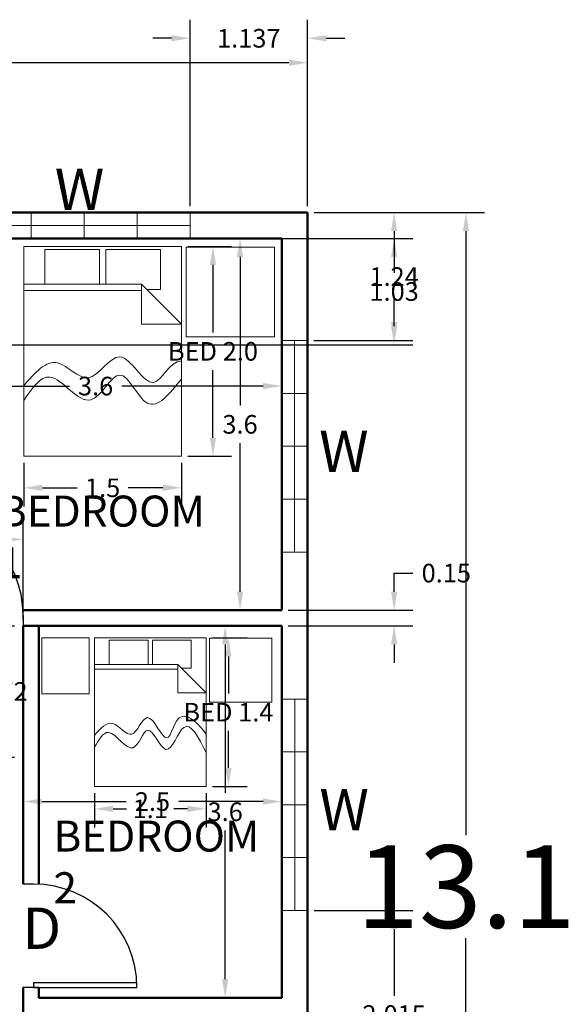
# Model space of a CAD drawing. Units: metres. Extents: x 3.9 to 21.3, y 24.8 to 56.5.
# Tile 6 of 6: x 13 to 18.3, y 31.2 to 40.8. Entities that reach past the tile are written whole.
import ezdxf

# ---------------------------------------------------------------- set-up
doc = ezdxf.new("R2010")
doc.units = ezdxf.units.M
doc.header["$MEASUREMENT"] = 0
for name, color, linetype, lineweight in [('A-AREA-IDEN', 3, 'Continuous', 25), ('DIMENSIONS', 2, 'Continuous', 18), ('DOOR', 5, 'Continuous', 25), ('FURNITURE', 6, 'Continuous', 18), ('TEXT', 3, 'Continuous', 18), ('WALL', 1, 'Continuous', 50), ('WINDOW', 4, 'Continuous', 18)]:
    doc.layers.add(name, color=color, linetype=linetype, lineweight=lineweight)
doc.styles.get("Standard").update_dxf_attribs({"font": 'arial.ttf'})
doc.dimstyles.get("Standard").update_dxf_attribs({"dimtxt": 0.18, "dimasz": 0.18, "dimexe": 0.18, "dimexo": 0.0625, "dimgap": 0.09, "dimtad": 0, "dimtih": 1, "dimtoh": 1, "dimdec": 1, "dimzin": 0, "dimdsep": 46, "dimtxsty": 'Standard', "dimcen": 0.09, "dimadec": 0, "dimazin": 0, "dimtfac": 1, "dimtdec": 1, "dimtofl": 0, "dimtmove": 0, "dimatfit": 3, "dimfxl": 1, "dimtolj": 1, "dimtzin": 0, "dimarcsym": 0})

# ---------------------------------------------------------------- blocks, each defined once
blk = doc.blocks.new('*U2')
for p, q in [((0, 0), (0, -100)), ((1000, 0), (1000, -100))]:
    blk.add_line(p, q)
blk.add_lwpolyline([(0, 0), (0, 1000), (43.75, 1000), (43.75, 0)], close=True)
blk.add_arc((0, 0), 1000, 0, 90)
blk = doc.blocks.new('Bed - Queen')
for p, q in [((0, -80.00003), (0, 0)), ((0, 0), (59.99999, 0)), ((59.99999, 0), (59.99999, -80.00003)), ((7.99999, -1.2), (28.79998, -1.2)), ((7.99999, -14.4), (7.99999, -1.2)), ((28.79998, -1.2), (28.79998, -14.4)), ((31.19999, -1.2), (51.99999, -1.2)), ((31.19999, -14.4), (31.19999, -1.2)), ((51.99999, -1.2), (51.99999, -16.4)), ((0, -14.4), (44.8, -14.4)), ((59.99999, -29.6), (44.8, -14.4)), ((44.8, -14.4), (44.8, -29.6)), ((44.8, -16.8), (0, -16.8)), ((51.99999, -16.4), (46.79936, -16.4)), ((44.8, -29.6), (59.99999, -29.6)), ((59.99999, -80.00003), (0, -80.00003))]:
    blk.add_line(p, q)
blk = doc.blocks.new('*U10')
for p, q in [((0, 0), (0, -100)), ((-1000, 0), (-1000, -100))]:
    blk.add_line(p, q)
blk.add_lwpolyline([(0, 0), (0, 1000), (-43.75, 1000), (-43.75, 0)], close=True)
blk.add_arc((0, 0), 1000, 90, 180)
blk = doc.blocks.new('*D21')
at = {"layer": 'Defpoints', "color": 0, "transparency": 16777216}
for p in [(15.7571, 38.8951), (15.7571, 25.8451), (17.2883, 25.8451)]:
    blk.add_point(p, dxfattribs=at)
at = {"layer": 'DIMENSIONS', "color": 0, "lineweight": -2, "transparency": 16777216}
for p, q in [((15.8196, 38.8951), (17.4683, 38.8951)), ((17.2883, 38.7151), (17.2883, 32.8688)), ((17.2883, 26.0251), (17.2883, 31.8713)), ((15.8196, 25.8451), (17.4683, 25.8451))]:
    blk.add_line(p, q, dxfattribs=at)
at = {"layer": 'DIMENSIONS', "color": 0, "transparency": 16777216}
for points in [[(17.2583, 38.7151), (17.3183, 38.7151), (17.2883, 38.8951)], [(17.2583, 26.0251), (17.3183, 26.0251), (17.2883, 25.8451)]]:
    blk.add_solid(points, dxfattribs=at)
at = {"layer": 'DIMENSIONS', "color": 0, "transparency": 16777216, "insert": (17.2883, 32.3701), "char_height": 0.18, "attachment_point": 5}
blk.add_mtext('\\A1;{\\H4.44444x;13.1}', dxfattribs=at)
blk = doc.blocks.new('*D22')
at = {"layer": 'Defpoints', "color": 0, "transparency": 16777216}
for p in [(15.7571, 40.3451), (6.1571, 38.8951), (15.7571, 38.8951)]:
    blk.add_point(p, dxfattribs=at)
at = {"layer": 'DIMENSIONS', "color": 0, "lineweight": -2, "transparency": 16777216}
for p, q in [((6.1571, 38.9576), (6.1571, 40.5251)), ((15.7571, 38.9576), (15.7571, 40.5251)), ((6.3371, 40.3451), (10.1392, 40.3451)), ((15.5771, 40.3451), (11.7751, 40.3451))]:
    blk.add_line(p, q, dxfattribs=at)
at = {"layer": 'DIMENSIONS', "color": 0, "transparency": 16777216}
for points in [[(6.3371, 40.3751), (6.3371, 40.3151), (6.1571, 40.3451)], [(15.5771, 40.3751), (15.5771, 40.3151), (15.7571, 40.3451)]]:
    blk.add_solid(points, dxfattribs=at)
at = {"layer": 'DIMENSIONS', "color": 0, "transparency": 16777216, "insert": (10.9571, 40.3451), "char_height": 0.18, "attachment_point": 5}
blk.add_mtext('\\A1;{\\H4.44444x;9.6}', dxfattribs=at)
blk = doc.blocks.new('*D25')
at = {"layer": 'Defpoints', "color": 0, "transparency": 16777216}
for p in [(11.9071, 37.772), (15.5071, 37.772), (15.5071, 37.2152)]:
    blk.add_point(p, dxfattribs=at)
at = {"layer": 'DIMENSIONS', "color": 0, "lineweight": -2, "transparency": 16777216}
for p, q in [((11.9071, 37.7095), (11.9071, 37.0352)), ((15.5071, 37.7095), (15.5071, 37.0352)), ((12.0871, 37.2152), (13.4534, 37.2152)), ((15.3271, 37.2152), (13.9609, 37.2152))]:
    blk.add_line(p, q, dxfattribs=at)
at = {"layer": 'DIMENSIONS', "color": 0, "transparency": 16777216}
for points in [[(12.0871, 37.2452), (12.0871, 37.1852), (11.9071, 37.2152)], [(15.3271, 37.2452), (15.3271, 37.1852), (15.5071, 37.2152)]]:
    blk.add_solid(points, dxfattribs=at)
at = {"layer": 'DIMENSIONS', "color": 0, "transparency": 16777216, "insert": (13.7071, 37.2152), "char_height": 0.18, "attachment_point": 5}
blk.add_mtext('\\A1;3.6', dxfattribs=at)
blk = doc.blocks.new('*D26')
at = {"layer": 'Defpoints', "color": 0, "transparency": 16777216}
for p in [(14.878, 38.6451), (14.9391, 35.0451), (15.1038, 35.0451)]:
    blk.add_point(p, dxfattribs=at)
at = {"layer": 'DIMENSIONS', "color": 0, "lineweight": -2, "transparency": 16777216}
for p, q in [((14.9405, 38.6451), (15.2838, 38.6451)), ((15.1038, 38.4651), (15.1038, 37.027)), ((15.1038, 35.2251), (15.1038, 36.6631)), ((15.0016, 35.0451), (15.2838, 35.0451))]:
    blk.add_line(p, q, dxfattribs=at)
at = {"layer": 'DIMENSIONS', "color": 0, "transparency": 16777216}
for points in [[(15.0738, 38.4651), (15.1338, 38.4651), (15.1038, 38.6451)], [(15.0738, 35.2251), (15.1338, 35.2251), (15.1038, 35.0451)]]:
    blk.add_solid(points, dxfattribs=at)
at = {"layer": 'DIMENSIONS', "color": 0, "transparency": 16777216, "insert": (15.1038, 36.8451), "char_height": 0.18, "attachment_point": 5}
blk.add_mtext('\\A1;3.6', dxfattribs=at)
blk = doc.blocks.new('*D28')
at = {"layer": 'Defpoints', "color": 0, "transparency": 16777216}
for p in [(13.0071, 33.4184), (15.5071, 33.4184), (13.0071, 33.1938)]:
    blk.add_point(p, dxfattribs=at)
at = {"layer": 'DIMENSIONS', "color": 0, "lineweight": -2, "transparency": 16777216}
for p, q in [((13.0071, 33.3559), (13.0071, 33.0138)), ((15.5071, 33.3559), (15.5071, 33.0138)), ((13.1871, 33.1938), (14.0011, 33.1938)), ((15.3271, 33.1938), (14.5132, 33.1938))]:
    blk.add_line(p, q, dxfattribs=at)
at = {"layer": 'DIMENSIONS', "color": 0, "transparency": 16777216}
for points in [[(13.1871, 33.2238), (13.1871, 33.1638), (13.0071, 33.1938)], [(15.3271, 33.2238), (15.3271, 33.1638), (15.5071, 33.1938)]]:
    blk.add_solid(points, dxfattribs=at)
at = {"layer": 'DIMENSIONS', "color": 0, "transparency": 16777216, "insert": (14.2571, 33.1938), "char_height": 0.18, "attachment_point": 5}
blk.add_mtext('\\A1;2.5', dxfattribs=at)
blk = doc.blocks.new('*D29')
at = {"layer": 'Defpoints', "color": 0, "transparency": 16777216}
for p in [(15.5071, 34.8951), (14.9602, 31.2951), (15.5071, 31.2951)]:
    blk.add_point(p, dxfattribs=at)
at = {"layer": 'DIMENSIONS', "color": 0, "lineweight": -2, "transparency": 16777216}
for p, q in [((15.4446, 34.8951), (14.7802, 34.8951)), ((14.9602, 34.7151), (14.9602, 33.277)), ((14.9602, 31.4751), (14.9602, 32.9131)), ((15.4446, 31.2951), (14.7802, 31.2951))]:
    blk.add_line(p, q, dxfattribs=at)
at = {"layer": 'DIMENSIONS', "color": 0, "transparency": 16777216}
for points in [[(14.9302, 34.7151), (14.9902, 34.7151), (14.9602, 34.8951)], [(14.9302, 31.4751), (14.9902, 31.4751), (14.9602, 31.2951)]]:
    blk.add_solid(points, dxfattribs=at)
at = {"layer": 'DIMENSIONS', "color": 0, "transparency": 16777216, "insert": (14.9602, 33.0951), "char_height": 0.18, "attachment_point": 5}
blk.add_mtext('\\A1;3.6', dxfattribs=at)
blk = doc.blocks.new('WIN-4-LIGHT-2046')
for p, q in [((0.5115, -0.125), (0, -0.125)), ((0.5115, -0.125), (1.0231, -0.125)), ((1.5346, -0.125), (1.0231, -0.125)), ((1.5346, -0.125), (2.0462, -0.125))]:
    blk.add_line(p, q)
for points in [[(0.5115, 0), (0, 0), (0, -0.25), (0.5115, -0.25)], [(0.5115, 0), (1.0231, 0), (1.0231, -0.25), (0.5115, -0.25)], [(1.5346, 0), (1.0231, 0), (1.0231, -0.25), (1.5346, -0.25)], [(1.5346, 0), (2.0462, 0), (2.0462, -0.25), (1.5346, -0.25)]]:
    blk.add_lwpolyline(points, close=True)
blk = doc.blocks.new('*D39')
at = {"layer": 'Defpoints', "color": 0, "transparency": 16777216}
for p in [(14.537, 38.5674), (14.8418, 38.5674), (14.537, 36.5354)]:
    blk.add_point(p, dxfattribs=at)
at = {"layer": 'DIMENSIONS', "color": 0, "lineweight": -2, "transparency": 16777216}
for p, q in [((14.5995, 38.5674), (15.0218, 38.5674)), ((14.8418, 38.3874), (14.8418, 37.7333)), ((14.8418, 36.7154), (14.8418, 37.3695)), ((14.5995, 36.5354), (15.0218, 36.5354))]:
    blk.add_line(p, q, dxfattribs=at)
at = {"layer": 'DIMENSIONS', "color": 0, "transparency": 16777216}
for points in [[(14.8118, 38.3874), (14.8718, 38.3874), (14.8418, 38.5674)], [(14.8118, 36.7154), (14.8718, 36.7154), (14.8418, 36.5354)]]:
    blk.add_solid(points, dxfattribs=at)
at = {"layer": 'DIMENSIONS', "color": 0, "transparency": 16777216, "insert": (14.8418, 37.5514), "char_height": 0.18, "attachment_point": 5}
blk.add_mtext('\\A1;BED 2.0', dxfattribs=at)
blk = doc.blocks.new('*D40')
at = {"layer": 'Defpoints', "color": 0, "transparency": 16777216}
for p in [(13.013, 36.5354), (14.537, 36.5354), (14.537, 36.2306)]:
    blk.add_point(p, dxfattribs=at)
at = {"layer": 'DIMENSIONS', "color": 0, "lineweight": -2, "transparency": 16777216}
for p, q in [((13.013, 36.4729), (13.013, 36.0506)), ((14.537, 36.4729), (14.537, 36.0506)), ((13.193, 36.2306), (13.529, 36.2306)), ((14.357, 36.2306), (14.0211, 36.2306))]:
    blk.add_line(p, q, dxfattribs=at)
at = {"layer": 'DIMENSIONS', "color": 0, "transparency": 16777216}
for points in [[(13.193, 36.2606), (13.193, 36.2006), (13.013, 36.2306)], [(14.357, 36.2606), (14.357, 36.2006), (14.537, 36.2306)]]:
    blk.add_solid(points, dxfattribs=at)
at = {"layer": 'DIMENSIONS', "color": 0, "transparency": 16777216, "insert": (13.775, 36.2306), "char_height": 0.18, "attachment_point": 5}
blk.add_mtext('\\A1;1.5', dxfattribs=at)
blk = doc.blocks.new('*D41')
at = {"layer": 'Defpoints', "color": 0, "transparency": 16777216}
for p in [(14.7753, 34.7785), (14.9913, 34.7785), (14.7753, 33.339)]:
    blk.add_point(p, dxfattribs=at)
at = {"layer": 'DIMENSIONS', "color": 0, "lineweight": -2, "transparency": 16777216}
for p, q in [((14.8378, 34.7785), (15.1713, 34.7785)), ((14.9913, 34.5985), (14.9913, 34.2392)), ((14.9913, 33.519), (14.9913, 33.8783)), ((14.8378, 33.339), (15.1713, 33.339))]:
    blk.add_line(p, q, dxfattribs=at)
at = {"layer": 'DIMENSIONS', "color": 0, "transparency": 16777216}
for points in [[(14.9613, 34.5985), (15.0213, 34.5985), (14.9913, 34.7785)], [(14.9613, 33.519), (15.0213, 33.519), (14.9913, 33.339)]]:
    blk.add_solid(points, dxfattribs=at)
at = {"layer": 'DIMENSIONS', "color": 0, "transparency": 16777216, "insert": (14.9913, 34.0587), "char_height": 0.18, "attachment_point": 5}
blk.add_mtext('\\A1;BED 1.4', dxfattribs=at)
blk = doc.blocks.new('*D42')
at = {"layer": 'Defpoints', "color": 0, "transparency": 16777216}
for p in [(13.6957, 33.339), (14.7753, 33.339), (14.7753, 33.1231)]:
    blk.add_point(p, dxfattribs=at)
at = {"layer": 'DIMENSIONS', "color": 0, "lineweight": -2, "transparency": 16777216}
for p, q in [((13.6957, 33.2765), (13.6957, 32.9431)), ((14.7753, 33.2765), (14.7753, 32.9431)), ((13.8757, 33.1231), (14.0075, 33.1231)), ((14.5953, 33.1231), (14.4635, 33.1231))]:
    blk.add_line(p, q, dxfattribs=at)
at = {"layer": 'DIMENSIONS', "color": 0, "transparency": 16777216}
for points in [[(13.8757, 33.1531), (13.8757, 33.0931), (13.6957, 33.1231)], [(14.5953, 33.1531), (14.5953, 33.0931), (14.7753, 33.1231)]]:
    blk.add_solid(points, dxfattribs=at)
at = {"layer": 'DIMENSIONS', "color": 0, "transparency": 16777216, "insert": (14.2355, 33.1231), "char_height": 0.18, "attachment_point": 5}
blk.add_mtext('\\A1;1.1', dxfattribs=at)
blk = doc.blocks.new('*D75')
at = {"layer": 'Defpoints', "color": 0, "transparency": 16777216}
for p in [(13.0071, 35.7316), (11.9071, 34.8951), (13.0071, 34.8951)]:
    blk.add_point(p, dxfattribs=at)
at = {"layer": 'DIMENSIONS', "color": 0, "lineweight": -2, "transparency": 16777216}
for p, q in [((11.9071, 34.9576), (11.9071, 35.9116)), ((13.0071, 34.9576), (13.0071, 35.9116)), ((12.0871, 35.7316), (12.2291, 35.7316)), ((12.8271, 35.7316), (12.6851, 35.7316))]:
    blk.add_line(p, q, dxfattribs=at)
at = {"layer": 'DIMENSIONS', "color": 0, "transparency": 16777216}
for points in [[(12.0871, 35.7616), (12.0871, 35.7016), (11.9071, 35.7316)], [(12.8271, 35.7616), (12.8271, 35.7016), (13.0071, 35.7316)]]:
    blk.add_solid(points, dxfattribs=at)
at = {"layer": 'DIMENSIONS', "color": 0, "transparency": 16777216, "insert": (12.4571, 35.7316), "char_height": 0.18, "attachment_point": 5}
blk.add_mtext('\\A1;1.1', dxfattribs=at)
blk = doc.blocks.new('*D86')
at = {"layer": 'Defpoints', "color": 0, "transparency": 16777216}
for p in [(15.7571, 40.5816), (14.62, 38.8951), (15.7571, 38.8951)]:
    blk.add_point(p, dxfattribs=at)
at = {"layer": 'DIMENSIONS', "color": 0, "lineweight": -2, "transparency": 16777216}
for p, q in [((14.62, 38.9576), (14.62, 40.7616)), ((15.7571, 38.9576), (15.7571, 40.7616)), ((14.44, 40.5816), (14.26, 40.5816)), ((15.9371, 40.5816), (16.1171, 40.5816))]:
    blk.add_line(p, q, dxfattribs=at)
at = {"layer": 'DIMENSIONS', "color": 0, "transparency": 16777216}
for points in [[(14.44, 40.6116), (14.44, 40.5516), (14.62, 40.5816)], [(15.9371, 40.6116), (15.9371, 40.5516), (15.7571, 40.5816)]]:
    blk.add_solid(points, dxfattribs=at)
at = {"layer": 'DIMENSIONS', "color": 0, "transparency": 16777216, "insert": (15.1886, 40.5816), "char_height": 0.18, "attachment_point": 5}
blk.add_mtext('\\A1;1.137', dxfattribs=at)
blk = doc.blocks.new('*D87')
at = {"layer": 'Defpoints', "color": 0, "transparency": 16777216}
for p in [(15.7571, 38.8951), (15.7547, 37.6552), (16.5936, 37.6552)]:
    blk.add_point(p, dxfattribs=at)
at = {"layer": 'DIMENSIONS', "color": 0, "lineweight": -2, "transparency": 16777216}
for p, q in [((15.8196, 38.8951), (16.7736, 38.8951)), ((16.5936, 38.7151), (16.5936, 38.4555)), ((16.5936, 37.8352), (16.5936, 38.0947)), ((15.8172, 37.6552), (16.7736, 37.6552))]:
    blk.add_line(p, q, dxfattribs=at)
at = {"layer": 'DIMENSIONS', "color": 0, "transparency": 16777216}
for points in [[(16.5636, 38.7151), (16.6236, 38.7151), (16.5936, 38.8951)], [(16.5636, 37.8352), (16.6236, 37.8352), (16.5936, 37.6552)]]:
    blk.add_solid(points, dxfattribs=at)
at = {"layer": 'DIMENSIONS', "color": 0, "transparency": 16777216, "insert": (16.5936, 38.2751), "char_height": 0.18, "attachment_point": 5}
blk.add_mtext('\\A1;1.24', dxfattribs=at)
blk = doc.blocks.new('*D90')
at = {"layer": 'Defpoints', "color": 0, "transparency": 16777216}
for p in [(15.7571, 32.1396), (16.5936, 32.1396), (15.7571, 30.1245)]:
    blk.add_point(p, dxfattribs=at)
at = {"layer": 'DIMENSIONS', "color": 0, "lineweight": -2, "transparency": 16777216}
for p, q in [((15.8196, 32.1396), (16.7736, 32.1396)), ((16.5936, 31.9596), (16.5936, 31.3139)), ((16.5936, 30.3045), (16.5936, 30.9501)), ((15.8196, 30.1245), (16.7736, 30.1245))]:
    blk.add_line(p, q, dxfattribs=at)
at = {"layer": 'DIMENSIONS', "color": 0, "transparency": 16777216}
for points in [[(16.5636, 31.9596), (16.6236, 31.9596), (16.5936, 32.1396)], [(16.5636, 30.3045), (16.6236, 30.3045), (16.5936, 30.1245)]]:
    blk.add_solid(points, dxfattribs=at)
at = {"layer": 'DIMENSIONS', "color": 0, "transparency": 16777216, "insert": (16.5936, 31.132), "char_height": 0.18, "attachment_point": 5}
blk.add_mtext('\\A1;2.015', dxfattribs=at)
blk = doc.blocks.new('*D93')
at = {"layer": 'Defpoints', "color": 0, "transparency": 16777216}
for p in [(15.5071, 35.0451), (16.5936, 35.0451), (15.5071, 34.8951)]:
    blk.add_point(p, dxfattribs=at)
at = {"layer": 'DIMENSIONS', "color": 0, "lineweight": -2, "transparency": 16777216}
for p, q in [((16.5936, 35.2251), (16.5936, 35.4051)), ((16.5936, 35.4051), (16.7736, 35.4051)), ((15.5696, 35.0451), (16.7736, 35.0451)), ((15.5696, 34.8951), (16.7736, 34.8951)), ((16.5936, 34.7151), (16.5936, 34.5351))]:
    blk.add_line(p, q, dxfattribs=at)
at = {"layer": 'DIMENSIONS', "color": 0, "transparency": 16777216}
for points in [[(16.5636, 35.2251), (16.6236, 35.2251), (16.5936, 35.0451)], [(16.5636, 34.7151), (16.6236, 34.7151), (16.5936, 34.8951)]]:
    blk.add_solid(points, dxfattribs=at)
at = {"layer": 'DIMENSIONS', "color": 0, "transparency": 16777216, "insert": (17.0981, 35.4051), "char_height": 0.18, "attachment_point": 5}
blk.add_mtext('\\A1;0.15', dxfattribs=at)
blk = doc.blocks.new('*D100')
at = {"layer": 'Defpoints', "color": 0, "transparency": 16777216}
for p in [(8.1743, 38.6451), (16.5936, 38.6451), (8.1743, 37.6158)]:
    blk.add_point(p, dxfattribs=at)
at = {"layer": 'DIMENSIONS', "color": 0, "lineweight": -2, "transparency": 16777216}
for p, q in [((8.2368, 38.6451), (16.7736, 38.6451)), ((16.5936, 38.4651), (16.5936, 38.3124)), ((16.5936, 37.7958), (16.5936, 37.9485)), ((8.2368, 37.6158), (16.7736, 37.6158))]:
    blk.add_line(p, q, dxfattribs=at)
at = {"layer": 'DIMENSIONS', "color": 0, "transparency": 16777216}
for points in [[(16.5636, 38.4651), (16.6236, 38.4651), (16.5936, 38.6451)], [(16.5636, 37.7958), (16.6236, 37.7958), (16.5936, 37.6158)]]:
    blk.add_solid(points, dxfattribs=at)
at = {"layer": 'DIMENSIONS', "color": 0, "transparency": 16777216, "insert": (16.5936, 38.1304), "char_height": 0.18, "attachment_point": 5}
blk.add_mtext('\\A1;1.03', dxfattribs=at)
blk = doc.blocks.new('*D102')
at = {"layer": 'Defpoints', "color": 0, "transparency": 16777216}
for p in [(11.9071, 34.8951), (11.9071, 33.623), (12.7436, 33.623)]:
    blk.add_point(p, dxfattribs=at)
at = {"layer": 'DIMENSIONS', "color": 0, "lineweight": -2, "transparency": 16777216}
for p, q in [((11.9696, 34.8951), (12.9236, 34.8951)), ((12.7436, 34.7151), (12.7436, 34.4394)), ((12.7436, 33.803), (12.7436, 34.0787)), ((11.9696, 33.623), (12.9236, 33.623))]:
    blk.add_line(p, q, dxfattribs=at)
at = {"layer": 'DIMENSIONS', "color": 0, "transparency": 16777216}
for points in [[(12.7136, 34.7151), (12.7736, 34.7151), (12.7436, 34.8951)], [(12.7136, 33.803), (12.7736, 33.803), (12.7436, 33.623)]]:
    blk.add_solid(points, dxfattribs=at)
at = {"layer": 'DIMENSIONS', "color": 0, "transparency": 16777216, "insert": (12.7436, 34.2591), "char_height": 0.18, "attachment_point": 5}
blk.add_mtext('\\A1;1.272', dxfattribs=at)

msp = doc.modelspace()

# ---------------------------------------------------------------- linework, layer by layer
at = {"layer": 'DOOR'}
msp.add_line((13.1571, 31.3951), (13.0071, 31.3951), dxfattribs=at)
at = {"layer": 'FURNITURE'}
for points in [[(14.5844, 38.5607), (15.4366, 38.5607), (15.4366, 37.6904), (14.5844, 37.6904)], [(13.6446, 34.7788), (13.1887, 34.7788), (13.1887, 34.2366), (13.6446, 34.2366)], [(14.8089, 34.7737), (15.4126, 34.7737), (15.4126, 34.1572), (14.8089, 34.1572)]]:
    msp.add_lwpolyline(points, close=True, dxfattribs=at)
for points, knots in [([(13.013, 37.2185), (13.1199, 37.344), (13.3142, 37.5725), (13.6547, 37.1383), (13.9505, 37.7181), (14.2608, 37.0266), (14.4234, 37.4587), (14.5379, 37.4585), (14.5383, 37.4585)], [0, 0, 0, 0, 0.396973, 0.72226, 1.087846, 1.495598, 1.837456, 1.838674, 1.838674, 1.838674, 1.838674]), ([(13.013, 37.0757), (13.0929, 37.1942), (13.2795, 37.4709), (13.6528, 36.8507), (13.949, 37.5395), (14.1999, 36.8621), (14.4224, 37.1402), (14.537, 37.2833)], [0, 0, 0, 0, 0.339288, 0.792781, 1.161072, 1.542093, 1.946429, 1.946429, 1.946429, 1.946429]), ([(13.6957, 33.8339), (13.7537, 33.9004), (13.8685, 34.0319), (14.0712, 33.7278), (14.2093, 34.1769), (14.4181, 33.6142), (14.4841, 34.1562), (14.7198, 33.9339), (14.7753, 33.8441)], [0, 0, 0, 0, 0.21241, 0.420171, 0.6408, 0.913652, 1.16981, 1.388488, 1.388488, 1.388488, 1.388488]), ([(13.6957, 33.7191), (13.7382, 33.7937), (13.8405, 33.9736), (14.0758, 33.556), (14.2101, 34.0429), (14.3998, 33.5166), (14.5657, 34.0854), (14.7017, 33.8158), (14.7753, 33.6699)], [0, 0, 0, 0, 0.198868, 0.47911, 0.69769, 0.953134, 1.227437, 1.551242, 1.551242, 1.551242, 1.551242])]:
    msp.add_open_spline(points, degree=3, knots=knots, dxfattribs=at)
at = {"layer": 'WALL'}
for p, q in [((9.5071, 38.8951), (15.7571, 38.8951)), ((15.7571, 25.8451), (15.7571, 38.8951)), ((11.9071, 38.6451), (15.5071, 38.6451)), ((15.5071, 35.0451), (15.5071, 38.6451)), ((13.0059, 35.0451), (15.5071, 35.0451)), ((13.0071, 34.8951), (15.5071, 34.8951)), ((13.0071, 32.3951), (13.0071, 34.8951)), ((13.1571, 32.3938), (13.1571, 34.8951)), ((15.5071, 31.2951), (15.5071, 34.8951)), ((13.0071, 30.4651), (13.0071, 31.3951)), ((13.1571, 31.2951), (13.1571, 31.3951)), ((13.1571, 31.2951), (15.5071, 31.2951))]:
    msp.add_line(p, q, dxfattribs=at)

# ---------------------------------------------------------------- block references
at = {"layer": 'DOOR', "xscale": 0.001, "yscale": 0.001, "zscale": 0.001}
msp.add_blockref('*U2', (12.0071, 34.9951), dxfattribs=at)
at = {"layer": 'DOOR', "xscale": 0.001, "yscale": 0.001, "zscale": 0.001, "rotation": 270}
msp.add_blockref('*U10', (13.1071, 31.3951), dxfattribs=at)
at = {"layer": 'FURNITURE'}
for p, xscale, yscale, zscale in [((13.013, 38.5674), 0.0254, 0.0254, 0.0254), ((13.6957, 34.7785), 0.0179936394065877, 0.0179936394065877, 0.0179936394065877)]:
    msp.add_blockref('Bed - Queen', p, dxfattribs=dict(at, xscale=xscale, yscale=yscale, zscale=zscale))
at = {"layer": 'WINDOW'}
msp.add_blockref('WIN-4-LIGHT-2046', (12.5738, 38.8951), dxfattribs=at)
for p, rotation in [((15.7547, 37.6552), 269.9999999999998), ((15.7571, 34.1857), 270.0000000000003)]:
    msp.add_blockref('WIN-4-LIGHT-2046', p, dxfattribs=dict(at, rotation=rotation))

# ---------------------------------------------------------------- texts
at = {"layer": 'A-AREA-IDEN', "char_height": 0.3, "attachment_point": 1}
for s, insert in [('BEDROOM 1', (12.7722, 36.1551)), ('BEDROOM 2', (13.2999, 33.0096))]:
    msp.add_mtext_dynamic_manual_height_columns(s, width=1.45972, gutter_width=1, heights=[0], dxfattribs=dict(at, insert=insert))
at = {"layer": 'TEXT', "char_height": 0.4, "attachment_point": 1}
for s, insert in [('W', (13.3123, 39.3185)), ('W', (15.8684, 36.7848)), ('W', (15.8708, 33.3154)), ('D', (12.9987, 32.1676))]:
    msp.add_mtext_dynamic_manual_height_columns(s, width=0.69425, gutter_width=1, heights=[0], dxfattribs=dict(at, insert=insert))

# ---------------------------------------------------------------- dimensions: what is measured, and where the dimension line sits
at = {"layer": 'DIMENSIONS'}
dim = msp.add_linear_dim(base=(15.7571, 40.3451), p1=(6.1571, 38.8951), p2=(15.7571, 38.8951), text='{\\H4.44444x;<>}', dimstyle='Standard', override={"dimclrd": 0, "dimclre": 0, "dimclrt": 0}, dxfattribs=at)
dim.commit()
dim.dimension.update_dxf_attribs({"geometry": '*D22', "text_midpoint": (10.9571, 40.3451)})
for base, p1, p2, override, picture, middle in [((15.7571, 40.5816), (14.62, 38.8951), (15.7571, 38.8951), {"dimdec": 3, "dimlfac": 1, "dimrnd": 0, "dimzin": 0, "dimdsep": 46, "dimlunit": 2}, '*D86', (15.1886, 40.5816)), ((15.5071, 37.2152), (11.9071, 37.772), (15.5071, 37.772), {"dimclrd": 0, "dimclre": 0, "dimclrt": 0}, '*D25', (13.7071, 37.2152)), ((14.537, 36.2306), (13.013, 36.5354), (14.537, 36.5354), {"dimdec": 1, "dimlfac": 1, "dimrnd": 0, "dimzin": 0, "dimdsep": 46, "dimlunit": 2}, '*D40', (13.775, 36.2306)), ((13.0071, 35.7316), (11.9071, 34.8951), (13.0071, 34.8951), {"dimdec": 1, "dimlfac": 1, "dimrnd": 0, "dimzin": 0, "dimdsep": 46, "dimlunit": 2}, '*D75', (12.4571, 35.7316)), ((13.0071, 33.1938), (15.5071, 33.4184), (13.0071, 33.4184), {"dimclrd": 0, "dimclre": 0, "dimclrt": 0}, '*D28', (14.2571, 33.1938)), ((14.7753, 33.1231), (13.6957, 33.339), (14.7753, 33.339), {"dimdec": 1, "dimlfac": 1, "dimrnd": 0, "dimzin": 0, "dimdsep": 46, "dimlunit": 2}, '*D42', (14.2355, 33.1231))]:
    dim = msp.add_linear_dim(base=base, p1=p1, p2=p2, dimstyle='Standard', override=override, dxfattribs=at)
    dim.commit()
    dim.dimension.update_dxf_attribs({"geometry": picture, "text_midpoint": middle})
for base, p1, p2, angle, override, picture, middle in [((16.5936, 37.6552), (15.7571, 38.8951), (15.7547, 37.6552), 90, {"dimdec": 2, "dimlfac": 1, "dimrnd": 0, "dimzin": 0, "dimdsep": 46, "dimlunit": 2}, '*D87', (16.5936, 38.2751)), ((16.5936, 38.6451), (8.1743, 37.6158), (8.1743, 38.6451), 90, {"dimdec": 2, "dimlfac": 1, "dimrnd": 0, "dimzin": 0, "dimdsep": 46, "dimlunit": 2}, '*D100', (16.5936, 38.1304)), ((15.1038, 35.0451), (14.878, 38.6451), (14.9391, 35.0451), 90, {"dimclrd": 0, "dimclre": 0, "dimclrt": 0}, '*D26', (15.1038, 36.8451)), ((16.5936, 35.0451), (15.5071, 34.8951), (15.5071, 35.0451), 90, {"dimdec": 2, "dimlfac": 1, "dimrnd": 0, "dimzin": 0, "dimdsep": 46, "dimlunit": 2}, '*D93', (17.0981, 35.4051)), ((12.7436, 33.623), (11.9071, 34.8951), (11.9071, 33.623), 270, {"dimdec": 3, "dimlfac": 1, "dimrnd": 0, "dimzin": 0, "dimdsep": 46, "dimlunit": 2}, '*D102', (12.7436, 34.2591)), ((14.9602, 31.2951), (15.5071, 34.8951), (15.5071, 31.2951), 90, {"dimclrd": 0, "dimclre": 0, "dimclrt": 0}, '*D29', (14.9602, 33.0951)), ((16.5936, 32.1396), (15.7571, 30.1245), (15.7571, 32.1396), 90, {"dimdec": 3, "dimlfac": 1, "dimrnd": 0, "dimzin": 0, "dimdsep": 46, "dimlunit": 2}, '*D90', (16.5936, 31.132))]:
    dim = msp.add_linear_dim(base=base, p1=p1, p2=p2, angle=angle, dimstyle='Standard', override=override, dxfattribs=at)
    dim.commit()
    dim.dimension.update_dxf_attribs({"geometry": picture, "text_midpoint": middle})
for base, p1, p2, text, override, picture, middle in [((17.2883128981, 25.8450722391), (15.7571276207, 38.8950722391), (15.7571276207, 25.8450722391), '{\\H4.44444x;<>}', {"dimclrd": 0, "dimclre": 0, "dimclrt": 0}, '*D21', (17.2883128981, 32.3700722391)), ((14.8418, 38.5674), (14.537, 36.5354), (14.537, 38.5674), 'BED <>', {"dimdec": 1, "dimlfac": 1, "dimrnd": 0, "dimzin": 0, "dimdsep": 46, "dimlunit": 2}, '*D39', (14.8418, 37.5514)), ((14.9913, 34.7785), (14.7753, 33.339), (14.7753, 34.7785), 'BED <>', {"dimdec": 1, "dimlfac": 1, "dimrnd": 0, "dimzin": 0, "dimdsep": 46, "dimlunit": 2}, '*D41', (14.9913, 34.0587))]:
    dim = msp.add_linear_dim(base=base, p1=p1, p2=p2, angle=90, text=text, dimstyle='Standard', override=override, dxfattribs=at)
    dim.commit()
    dim.dimension.update_dxf_attribs({"geometry": picture, "text_midpoint": middle})

doc.saveas('drawing.dxf')
